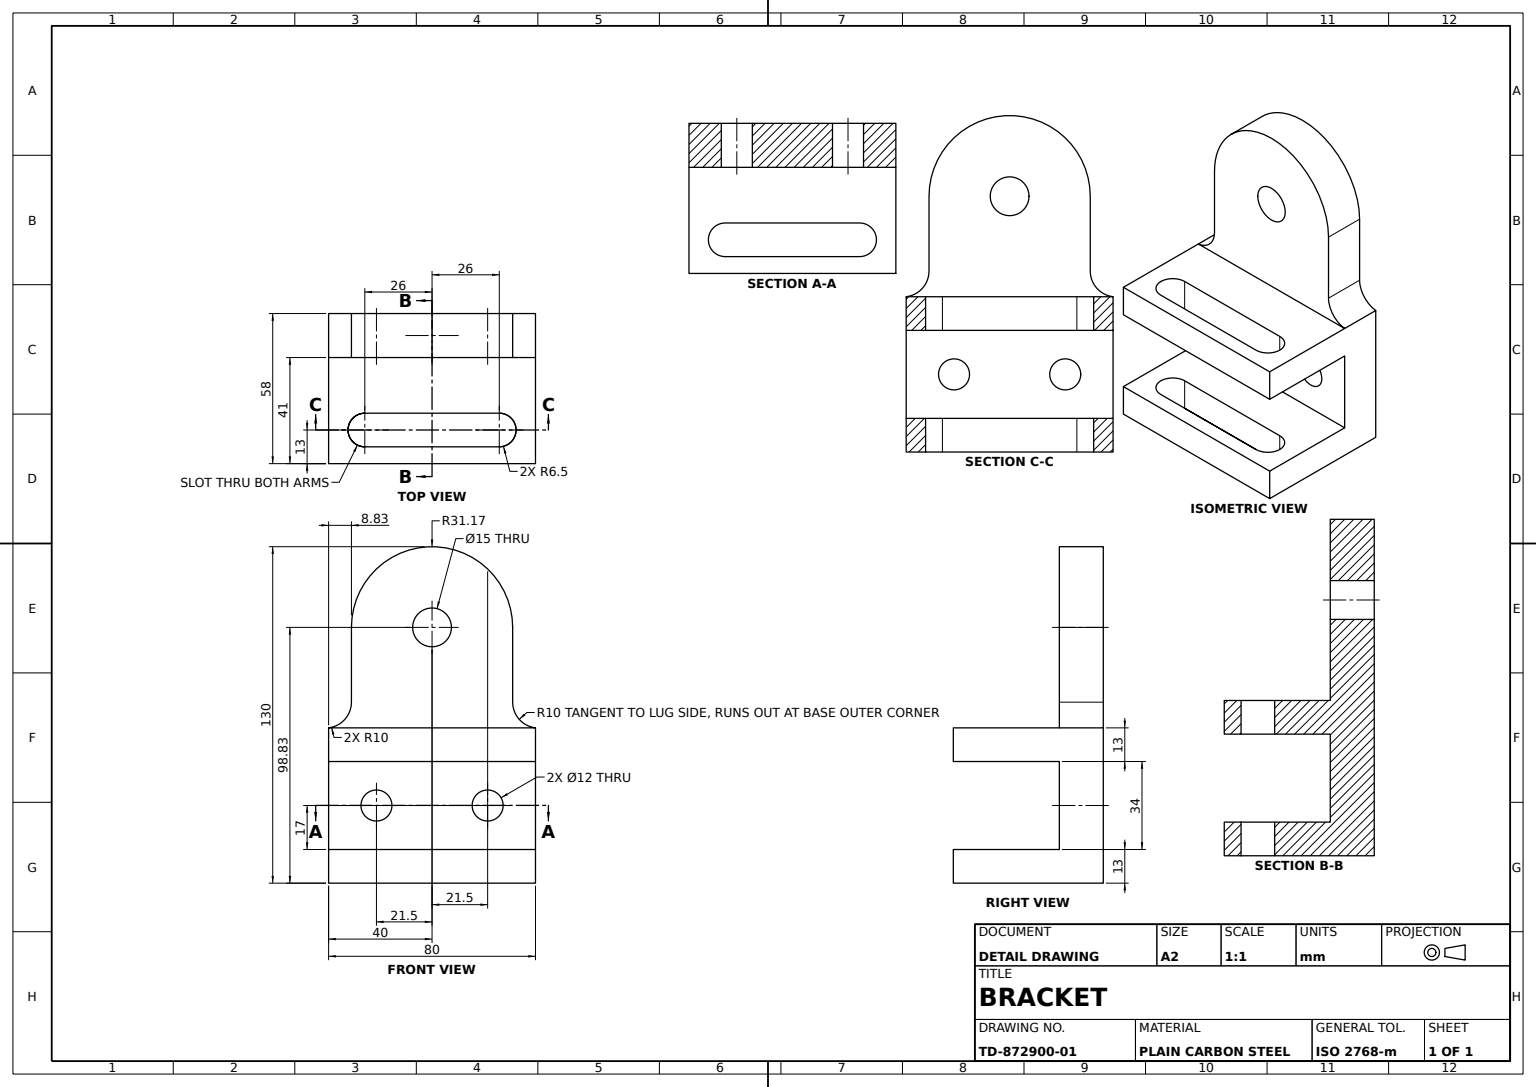
from build123d import *

# Parameters (mm, degrees)
BRACKET_BODY_DEPTH    = 40
ROUNDED_LUG_CUT_DEPTH = 80
PIN_HOLE_SKETCH_R     = 7.5
PIN_HOLE_15_DEPTH     = 80
FORK_GAP_SKETCH_R     = 6
FORK_GAP_12MM_DEPTH   = 80
ARM_SLOTS_2X6_5_DEPTH = 80


with BuildPart() as part:
    # Bracket Profile Sketch → Bracket Body (new, symmetric)
    with BuildSketch(Plane.XY):
        Polygon((0, 0), (58, 0), (58, 13), (17, 13), (17, 47), (58, 47), (58, 60), (17, 60), (17, 130), (0, 130), align=None)
    extrude(amount=BRACKET_BODY_DEPTH, both=True)

    # Lug Shape Sketch → Rounded Lug Cut (cut)
    with BuildSketch(Plane(origin=(17, 0, 0), x_dir=(0, 0, -1), z_dir=(1, 0, 0))):
        with BuildLine():
            Line((40, 130), (9.4e-08, 130))
            ThreePointArc((9.4e-08, 130), (22.043839272, 120.869142787), (31.174696418, 98.825303582))
            Line((31.174696418, 98.825303582), (31.174696418, 69.93076474))
            ThreePointArc((31.174696418, 69.93076474), (33.699839758, 63.287985359), (40, 60))
            Line((40, 60), (40, 130))
        make_face()
        with BuildLine():
            Line((-31.174696418, 69.93076474), (-31.174696418, 98.825303582))
            ThreePointArc((-31.174696418, 98.825303582), (-22.043839205, 120.869142854), (9.4e-08, 130))
            Line((9.4e-08, 130), (-40, 130))
            Line((-40, 130), (-40, 60))
            ThreePointArc((-40, 60), (-33.699839758, 63.287985359), (-31.174696418, 69.93076474))
        make_face()
    extrude(amount=-ROUNDED_LUG_CUT_DEPTH, mode=Mode.SUBTRACT)

    # Pin Hole Sketch → Pin Hole Ø15 (cut)
    with BuildSketch(Plane(origin=(17, 0, 0), x_dir=(0, 0, -1), z_dir=(1, 0, 0))):
        with Locations((0, 98.825303582)):
            Circle(PIN_HOLE_SKETCH_R)
    extrude(amount=-PIN_HOLE_15_DEPTH, mode=Mode.SUBTRACT)

    # Fork Gap Sketch → Fork Gap 12mm (cut)
    with BuildSketch(Plane(origin=(17, 0, 0), x_dir=(0, 0, -1), z_dir=(1, 0, 0))):
        with Locations((-21.5, 30)):
            Circle(FORK_GAP_SKETCH_R)
        with Locations((21.5, 30)):
            Circle(FORK_GAP_SKETCH_R)
    extrude(amount=-FORK_GAP_12MM_DEPTH, mode=Mode.SUBTRACT)

    # Arm Slots Sketch → Arm Slots 2x6.5 (cut)
    with BuildSketch(Plane(origin=(0, 60, 0), x_dir=(1, 0, 0), z_dir=(0, 1, 0))):
        with BuildLine():
            Line((38.5, -26), (38.5, 26))
            ThreePointArc((38.5, 26), (45, 32.5), (51.5, 26))
            Line((51.5, 26), (51.5, -26))
            ThreePointArc((51.5, -26), (45, -32.5), (38.5, -26))
        make_face()
    extrude(amount=-ARM_SLOTS_2X6_5_DEPTH, mode=Mode.SUBTRACT)


solid = part.part
